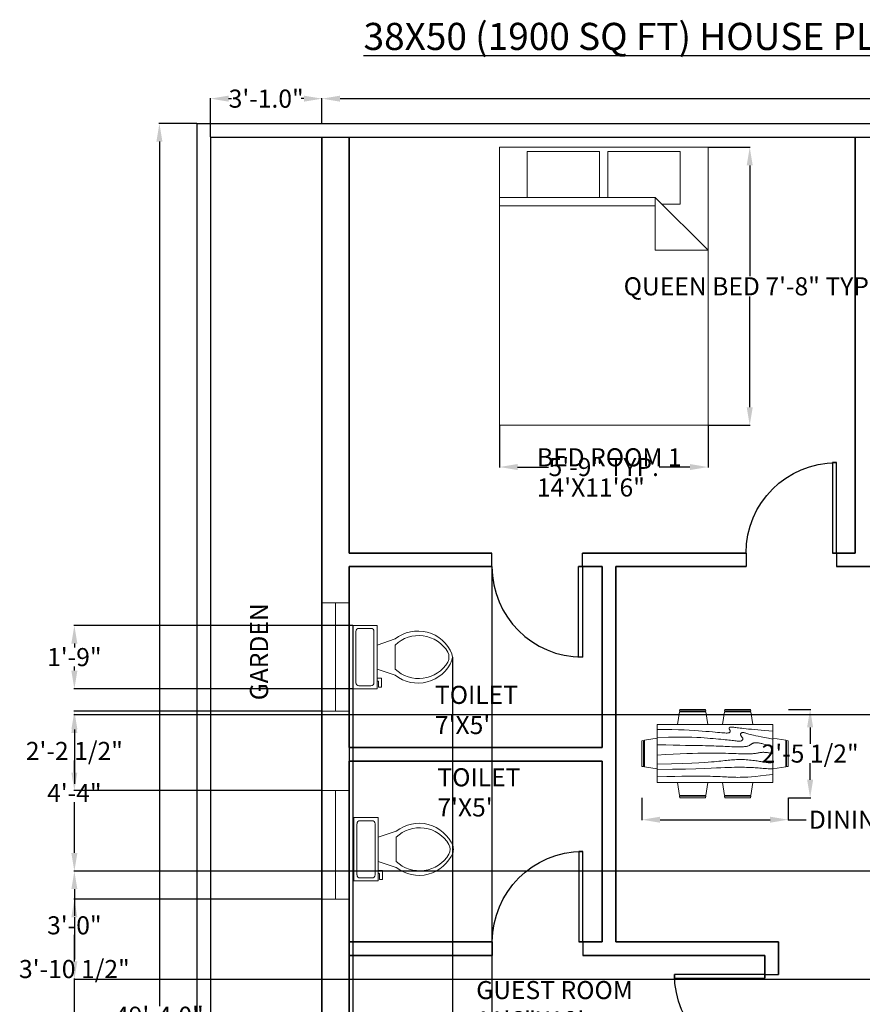
# Model space of a CAD drawing. Units: inches. Extents: x 889 to 1449, y 3224 to 3899.
# Tile 3 of 4: x 889 to 1169, y 3565 to 3892. Entities that reach past the tile are written whole.
import ezdxf

# ---------------------------------------------------------------- set-up
doc = ezdxf.new("R2010")
doc.units = ezdxf.units.IN
doc.header["$MEASUREMENT"] = 0
for name, color, linetype, lineweight in [('A-ANNO-DIMS', 2, 'Continuous', 18), ('A-ANNO-TEXT', 7, 'Continuous', 25), ('A-AREA-IDEN', 7, 'Continuous', 18), ('A-DOOR', 4, 'Continuous', 25), ('A-FLOR-FIXT', 9, 'Continuous', 18), ('A-FURN', 8, 'Continuous', 18), ('A-GLAZ', 4, 'Continuous', 18), ('A-WALL', 7, 'Continuous', 35), ('C-PROP', 7, 'Continuous', 25)]:
    doc.layers.add(name, color=color, linetype=linetype, lineweight=lineweight)
doc.styles.get("Standard").update_dxf_attribs({"font": 'arial.ttf'})
doc.dimstyles.get("Standard").update_dxf_attribs({"dimtxt": 6, "dimasz": 6, "dimexe": 0.18, "dimexo": 0.0625, "dimgap": 0.09, "dimtad": 0, "dimtih": 1, "dimtoh": 1, "dimdec": 1, "dimzin": 0, "dimdsep": 46, "dimlunit": 3, "dimtxsty": 'Standard', "dimcen": 0.09, "dimadec": 0, "dimazin": 0, "dimtfac": 1, "dimtdec": 1, "dimtofl": 0, "dimtmove": 0, "dimatfit": 3, "dimfxl": 1, "dimtolj": 1, "dimtzin": 0, "dimarcsym": 0})

# ---------------------------------------------------------------- blocks, each defined once
blk = doc.blocks.new('*U2')
for p, q in [((0, 0), (0, -6)), ((40, 0), (40, -6))]:
    blk.add_line(p, q)
blk.add_lwpolyline([(0, 0), (0, 40), (1.75, 40), (1.75, 0)], close=True)
blk.add_arc((0, 0), 40, 0, 90)
blk = doc.blocks.new('Dining Set - 36 x 72 in.')
for p, q in [((-22.2343, 26.00059), (-23.4847, 17.99762)), ((-22.2304, 26), (-5.7608, 26)), ((-22, 27.5), (-22.1562, 26.50042)), ((-5.8416, 26.5), (-22.1534, 26.5)), ((-22, 27.5), (-6, 27.5)), ((-5.8437, 26.49966), (-6, 27.5)), ((-4.5152, 17.99762), (-5.7655, 25.99926)), ((5.7657, 26.00059), (4.5153, 17.99762)), ((5.7696, 26), (22.2392, 26)), ((6, 27.5), (5.8438, 26.50042)), ((22.1584, 26.5), (5.8466, 26.5)), ((6, 27.5), (22, 27.5)), ((22.1563, 26.49966), (22, 27.5)), ((23.4848, 17.99762), (22.2345, 25.99926)), ((36, 18), (-36, 18)), ((-36, 18), (-36, -18)), ((36, -18), (36, 18)), ((-45.5, 8), (-44.5004, 8.15617)), ((-45.5, 8), (-45.5, -8)), ((-44.5, -8.15843), (-44.5, 8.15338)), ((-44.0006, 8.23428), (-35.9976, 9.48474)), ((-44, 8.23041), (-44, -8.23915)), ((44.0006, 8.23428), (35.9976, 9.48474)), ((44, 8.23041), (44, -8.23915)), ((44.5, -8.15843), (44.5, 8.15338)), ((45.5, 8), (44.5005, 8.15617)), ((45.5, 8), (45.5, -8)), ((-44.4997, -8.15631), (-45.5, -8)), ((-35.9976, -9.48476), (-43.9993, -8.2345)), ((35.9976, -9.48476), (43.9993, -8.2345)), ((44.4997, -8.15631), (45.5, -8)), ((-36, -18), (36, -18)), ((-22.2343, -26.0006), (-23.4847, -17.99762)), ((-4.5152, -17.99762), (-5.7655, -25.99928)), ((5.7657, -26.0006), (4.5153, -17.99762)), ((23.4848, -17.99762), (22.2345, -25.99928)), ((-22.2304, -26), (-5.7608, -26)), ((-22, -27.5), (-22.1562, -26.50044)), ((-5.8416, -26.5), (-22.1534, -26.5)), ((-22, -27.5), (-6, -27.5)), ((-5.8437, -26.49967), (-6, -27.5)), ((5.7696, -26), (22.2392, -26)), ((6, -27.5), (5.8438, -26.50044)), ((22.1584, -26.5), (5.8466, -26.5)), ((6, -27.5), (22, -27.5)), ((22.1563, -26.49967), (22, -27.5))]:
    blk.add_line(p, q)
for points in [[(-36, 15), (-31.1772, 14.97754), (-26.8079, 14.91406), (-22.8538, 14.81543), (-19.276, 14.6875), (-16.0362, 14.53613), (-13.0957, 14.36718), (-10.4159, 14.18652), (-7.9583, 14), (-5.6904, 13.81315), (-3.6035, 13.63021), (-1.6954, 13.45508), (0.0365, 13.29166), (1.5945, 13.14388), (2.9811, 13.01562), (4.1988, 12.9108), (5.25, 12.83333), (6.1393, 12.78613), (6.8802, 12.76823), (7.4883, 12.77767), (7.9792, 12.8125), (8.3685, 12.87077), (8.6719, 12.95052), (8.9049, 13.0498), (9.0833, 13.16666), (9.2205, 13.29899), (9.3216, 13.44401), (9.3895, 13.59879), (9.4271, 13.76041), (9.4373, 13.92594), (9.4232, 14.09245), (9.3875, 14.257), (9.3333, 14.41666), (9.2638, 14.56917), (9.1836, 14.71484), (9.0975, 14.85465), (9.0104, 14.98958), (8.9272, 15.1206), (8.8529, 15.2487), (8.7922, 15.37483), (8.75, 15.5), (8.7305, 15.62467), (8.7344, 15.74739), (8.7617, 15.86621), (8.8125, 15.97916), (8.8867, 16.08431), (8.9844, 16.17968), (9.1055, 16.26334), (9.25, 16.33333), (9.4189, 16.38802), (9.6172, 16.42708), (9.8506, 16.45052), (10.125, 16.45833), (10.4463, 16.45052), (10.8203, 16.42708), (11.2529, 16.38802), (11.75, 16.33333), (12.3184, 16.26318), (12.9694, 16.17838), (13.7151, 16.07991), (14.5677, 15.96875), (15.5395, 15.84586), (16.6426, 15.71224), (17.8893, 15.56884), (19.2917, 15.41666), (20.859, 15.25667), (22.5879, 15.08984), (24.4721, 14.91715), (26.5052, 14.73958), (28.6809, 14.5581), (30.9929, 14.3737), (33.4347, 14.18733), (36, 14)], [(-36, 10), (-28.9766, 10.14274), (-23.1725, 10.20442), (-18.4241, 10.19775), (-14.5677, 10.13541), (-11.4399, 10.03011), (-8.877, 9.89453), (-6.7154, 9.74137), (-4.7917, 9.58333), (-2.9698, 9.43082), (-1.2246, 9.28515), (0.4415, 9.14534), (2.026, 9.01041), (3.5266, 8.87939), (4.9408, 8.7513), (6.266, 8.62516), (7.5, 8.5), (8.6411, 8.37549), (9.6914, 8.2539), (10.6538, 8.13818), (11.5312, 8.03125), (12.3267, 7.93603), (13.043, 7.85547), (13.6831, 7.79248), (14.25, 7.75), (14.7471, 7.7303), (15.1797, 7.73307), (15.5537, 7.75732), (15.875, 7.80208), (16.1494, 7.86637), (16.3828, 7.94922), (16.5811, 8.04964), (16.75, 8.16666), (16.8944, 8.29915), (17.0143, 8.44531), (17.1089, 8.60319), (17.1771, 8.77083), (17.218, 8.94629), (17.2305, 9.1276), (17.2137, 9.31282), (17.1667, 9.5), (17.0895, 9.6875), (16.987, 9.875), (16.8649, 10.0625), (16.7292, 10.25), (16.5856, 10.4375), (16.4401, 10.625), (16.2985, 10.8125), (16.1667, 11), (16.05, 11.18733), (15.9518, 11.3737), (15.8752, 11.5581), (15.8229, 11.73958), (15.798, 11.91715), (15.8034, 12.08984), (15.842, 12.25667), (15.9167, 12.41666), (16.0295, 12.56836), (16.1784, 12.70833), (16.3605, 12.83268), (16.5729, 12.9375), (16.8127, 13.01888), (17.0768, 13.07291), (17.3625, 13.0957), (17.6667, 13.08333), (17.9894, 13.03312), (18.3418, 12.94726), (18.7382, 12.82918), (19.1927, 12.68229), (19.7195, 12.51001), (20.3327, 12.31575), (21.0465, 12.10294), (21.875, 11.875), (22.8357, 11.63354), (23.959, 11.37304), (25.2786, 11.08618), (26.8282, 10.76562), (28.6414, 10.40405), (30.752, 9.99414), (33.1936, 9.52856), (36, 9)], [(-36, 5.5), (-30.7157, 5.3348), (-26.069, 5.20963), (-21.9946, 5.11767), (-18.4271, 5.05208), (-15.3009, 5.00602), (-12.5508, 4.97265), (-10.1112, 4.94515), (-7.9167, 4.91666), (-5.909, 4.88167), (-4.0586, 4.83984), (-2.3429, 4.79215), (-0.7396, 4.73958), (0.7739, 4.6831), (2.22, 4.6237), (3.6213, 4.56233), (5, 4.5), (6.373, 4.43782), (7.7344, 4.3776), (9.0723, 4.32129), (10.375, 4.27083), (11.6309, 4.22819), (12.8281, 4.19531), (13.9551, 4.17415), (15, 4.16666), (15.954, 4.17448), (16.819, 4.19791), (17.6001, 4.23698), (18.3021, 4.29166), (18.9299, 4.36198), (19.4883, 4.44791), (19.9823, 4.54948), (20.4167, 4.66666), (20.7969, 4.79899), (21.1302, 4.94401), (21.4245, 5.09879), (21.6875, 5.26041), (21.9271, 5.42594), (22.1511, 5.59245), (22.3672, 5.757), (22.5834, 5.91666), (22.8065, 6.06868), (23.0404, 6.21093), (23.2879, 6.34147), (23.5521, 6.45833), (23.8358, 6.55957), (24.142, 6.64323), (24.4735, 6.70735), (24.8334, 6.75), (25.2235, 6.76969), (25.642, 6.76692), (26.0858, 6.74267), (26.5521, 6.69791), (27.0379, 6.63362), (27.5404, 6.55078), (28.0565, 6.45036), (28.5834, 6.33333), (29.1242, 6.19987), (29.7071, 6.04687), (30.3661, 5.87044), (31.1354, 5.66666), (32.0493, 5.43164), (33.142, 5.16146), (34.4475, 4.85221), (36, 4.5)], [(-36, -1), (-30.7915, -0.6591), (-26.0195, -0.38216), (-21.6519, -0.16284), (-17.6563, 0.00521), (-14.0005, 0.12833), (-10.6523, 0.21289), (-7.5796, 0.26522), (-4.75, 0.29166), (-2.134, 0.29793), (0.2878, 0.28711), (2.5317, 0.26163), (4.6146, 0.22396), (6.5529, 0.17651), (8.3633, 0.12174), (10.0623, 0.06209), (11.6667, 0), (13.1899, -0.06201), (14.6341, -0.1211), (15.9982, -0.17432), (17.2813, -0.21875), (18.4823, -0.25147), (19.6003, -0.26953), (20.6343, -0.27002), (21.5834, -0.25), (22.4481, -0.20768), (23.2357, -0.14584), (23.9549, -0.06836), (24.6146, 0.02083), (25.2235, 0.11784), (25.7904, 0.21875), (26.3241, 0.31966), (26.8334, 0.41666), (27.3265, 0.50618), (27.8099, 0.58593), (28.2894, 0.65397), (28.7709, 0.70833), (29.2601, 0.74707), (29.763, 0.76823), (30.2855, 0.76985), (30.8334, 0.75), (31.4088, 0.70784), (31.9994, 0.64713), (32.589, 0.57275), (33.1615, 0.48958), (33.7008, 0.4025), (34.1908, 0.3164), (34.6153, 0.23616), (34.9584, 0.16666), (35.2099, 0.11165), (35.3848, 0.07031), (35.504, 0.04069), (35.5886, 0.02083), (35.6594, 0.00879), (35.7377, 0.0026), (35.8442, 0.00032), (36, 0)], [(-36, -6.5), (-27.1843, -6.31267), (-20.084, -6.1263), (-14.469, -5.9419), (-10.1094, -5.76042), (-6.7752, -5.58285), (-4.2363, -5.41016), (-2.2629, -5.24333), (-0.625, -5.08334), (0.8708, -4.93099), (2.2715, -4.78646), (3.5872, -4.64974), (4.8281, -4.52084), (6.0046, -4.39974), (7.127, -4.28646), (8.2053, -4.18099), (9.25, -4.08334), (10.2705, -3.99382), (11.2734, -3.91407), (12.2647, -3.84603), (13.25, -3.79167), (14.2354, -3.75293), (15.2266, -3.73177), (16.2295, -3.73015), (17.25, -3.75), (18.2912, -3.79248), (19.3451, -3.85547), (20.4009, -3.93604), (21.4479, -4.03125), (22.4754, -4.13819), (23.4727, -4.25391), (24.4289, -4.37549), (25.3334, -4.5), (26.1785, -4.62492), (26.9694, -4.74935), (27.7145, -4.87281), (28.4219, -4.99479), (29.1, -5.11483), (29.7572, -5.23242), (30.4016, -5.34709), (31.0417, -5.45834), (31.6837, -5.56437), (32.3262, -5.65821), (32.9658, -5.73153), (33.599, -5.77604), (34.2224, -5.78345), (34.8327, -5.74545), (35.4264, -5.65373), (36, -5.5)], [(-36, -10), (-26.4022, -9.81299), (-18.4675, -9.62891), (-11.9839, -9.45069), (-6.7396, -9.28125), (-2.5226, -9.12354), (0.8789, -8.98047), (3.6769, -8.85498), (6.0833, -8.75), (8.2767, -8.66765), (10.3021, -8.60677), (12.1712, -8.56543), (13.8958, -8.54167), (15.4876, -8.53353), (16.9583, -8.53907), (18.3197, -8.55632), (19.5834, -8.58334), (20.7616, -8.61841), (21.8685, -8.66081), (22.9188, -8.71004), (23.9271, -8.76563), (24.9081, -8.82707), (25.8763, -8.89388), (26.8465, -8.96558), (27.8334, -9.04167), (28.8474, -9.12118), (29.8828, -9.20117), (30.93, -9.27824), (31.9792, -9.34896), (33.0205, -9.40991), (34.0443, -9.45768), (35.0407, -9.48885), (36, -9.5)], [(-36, -14.5), (-30.0881, -14.33513), (-25.0332, -14.21224), (-20.7312, -14.12647), (-17.0781, -14.07292), (-13.97, -14.04671), (-11.3027, -14.04297), (-8.9724, -14.05681), (-6.875, -14.08334), (-4.9224, -14.11833), (-3.0905, -14.16016), (-1.3709, -14.20785), (0.2448, -14.26042), (1.7647, -14.3169), (3.1973, -14.3763), (4.5507, -14.43767), (5.8333, -14.5), (7.0554, -14.5621), (8.235, -14.62175), (9.3922, -14.67652), (10.5469, -14.72396), (11.7192, -14.76164), (12.929, -14.78711), (14.1965, -14.79794), (15.5417, -14.79167), (16.9933, -14.76424), (18.6152, -14.70508), (20.4804, -14.60197), (22.6615, -14.44271), (25.2312, -14.21509), (28.2624, -13.9069), (31.8277, -13.50594), (36, -13)]]:
    blk.add_lwpolyline(points)
blk = doc.blocks.new('Bed - Queen')
for p, q in [((0, -80.00003), (0, 0)), ((0, 0), (59.99999, 0)), ((59.99999, 0), (59.99999, -80.00003)), ((7.99999, -1.2), (28.79998, -1.2)), ((7.99999, -14.4), (7.99999, -1.2)), ((28.79998, -1.2), (28.79998, -14.4)), ((31.19999, -1.2), (51.99999, -1.2)), ((31.19999, -14.4), (31.19999, -1.2)), ((51.99999, -1.2), (51.99999, -16.4)), ((0, -14.4), (44.8, -14.4)), ((44.8, -16.8), (0, -16.8)), ((59.99999, -29.6), (44.8, -14.4)), ((44.8, -14.4), (44.8, -29.6)), ((51.99999, -16.4), (46.79936, -16.4)), ((44.8, -29.6), (59.99999, -29.6)), ((59.99999, -80.00003), (0, -80.00003))]:
    blk.add_line(p, q)
blk = doc.blocks.new('*U15')
for p, q in [((9.5, -6), (9.5, -2)), ((-10, -8.5), (-8, -8.5)), ((-10, -9.5), (-10, -8.5)), ((-7, -9.5), (-10, -9.5)), ((-8, -8.5), (-8, -8)), ((-7, -8), (-7, -9.5)), ((-4, -8), (-6, -14)), ((4, -8), (6, -14)), ((4, -14), (-4, -14))]:
    blk.add_line(p, q)
blk.add_lwpolyline([(10.5, -8), (10.5, 0), (-10.5, 0), (-10.5, -8)], close=True)
for points in [[(-9.5, -2), (-9.5, -6)], [(8.5, -1), (-8.5, -1)], [(-8.5, -7), (8.5, -7)]]:
    blk.add_lwpolyline(points)
for centre, radius, start, end in [((-8.62, -1.88), 0.884, 81.8699, 188.1301), ((8.62, -1.88), 0.884, 351.8699, 98.1301), ((-8.62, -6.12), 0.884, 171.8699, 278.1301), ((8.62, -6.12), 0.884, 261.8699, 8.1301), ((3.52, -21.58), 12.17, 141.4691, 247.9714), ((4.2, -21.82), 11.33, 136.3677, 238.9468), ((-3.52, -21.58), 12.17, 292.0284, 38.5307), ((-4.2, -21.82), 11.33, 301.053, 43.6321), ((0, -27.88), 4, 245.7318, 294.2682), ((0, -29), 4, 254.8605, 285.1395)]:
    blk.add_arc(centre, radius, start, end)
blk = doc.blocks.new('*D17')
at = {"layer": 'A-ANNO-DIMS', "color": 0, "lineweight": -2, "transparency": 16777216}
for p, q in [((952.45, 3852.92), (952.45, 3865.8)), ((958.45, 3865.62), (959.39, 3865.62)), ((983.45, 3865.62), (982.5, 3865.62)), ((989.45, 3857.42), (989.45, 3865.8))]:
    blk.add_line(p, q, dxfattribs=at)
at = {"layer": 'A-ANNO-DIMS', "color": 0, "transparency": 16777216}
for points in [[(958.45, 3866.62), (958.45, 3864.62), (952.45, 3865.62)], [(983.45, 3866.62), (983.45, 3864.62), (989.45, 3865.62)]]:
    blk.add_solid(points, dxfattribs=at)
at = {"layer": 'Defpoints', "color": 0, "transparency": 16777216}
for p in [(989.45, 3865.62), (989.45, 3857.35), (952.45, 3852.85)]:
    blk.add_point(p, dxfattribs=at)
at = {"layer": 'A-ANNO-DIMS', "color": 0, "transparency": 16777216, "insert": (970.95, 3865.62), "char_height": 6, "attachment_point": 5}
blk.add_mtext('\\A1;3\'-1.0"', dxfattribs=at)
blk = doc.blocks.new('*D18')
at = {"layer": 'A-ANNO-DIMS', "color": 0, "lineweight": -2, "transparency": 16777216}
for p, q in [((989.45, 3857.42), (989.45, 3865.8)), ((995.45, 3865.62), (1181.06, 3865.62)), ((1394.45, 3865.62), (1208.83, 3865.62)), ((1400.45, 3857.42), (1400.45, 3865.8))]:
    blk.add_line(p, q, dxfattribs=at)
at = {"layer": 'A-ANNO-DIMS', "color": 0, "transparency": 16777216}
for points in [[(995.45, 3866.62), (995.45, 3864.62), (989.45, 3865.62)], [(1394.45, 3866.62), (1394.45, 3864.62), (1400.45, 3865.62)]]:
    blk.add_solid(points, dxfattribs=at)
at = {"layer": 'Defpoints', "color": 0, "transparency": 16777216}
for p in [(1400.45, 3865.62), (989.45, 3857.35), (1400.45, 3857.35)]:
    blk.add_point(p, dxfattribs=at)
at = {"layer": 'A-ANNO-DIMS', "color": 0, "transparency": 16777216, "insert": (1194.95, 3865.62), "char_height": 6, "attachment_point": 5}
blk.add_mtext('\\A1;34\'-3.0"', dxfattribs=at)
blk = doc.blocks.new('*D19')
at = {"layer": 'A-ANNO-DIMS', "color": 0, "lineweight": -2, "transparency": 16777216}
for p, q in [((947.88, 3857.35), (935.33, 3857.35)), ((935.51, 3851.35), (935.51, 3564.51)), ((935.51, 3271.35), (935.51, 3558.2)), ((947.88, 3265.35), (935.33, 3265.35))]:
    blk.add_line(p, q, dxfattribs=at)
at = {"layer": 'A-ANNO-DIMS', "color": 0, "transparency": 16777216}
for points in [[(934.51, 3851.35), (936.51, 3851.35), (935.51, 3857.35)], [(934.51, 3271.35), (936.51, 3271.35), (935.51, 3265.35)]]:
    blk.add_solid(points, dxfattribs=at)
at = {"layer": 'Defpoints', "color": 0, "transparency": 16777216}
for p in [(947.95, 3857.35), (935.51, 3265.35), (947.95, 3265.35)]:
    blk.add_point(p, dxfattribs=at)
at = {"layer": 'A-ANNO-DIMS', "color": 0, "transparency": 16777216, "insert": (935.51, 3561.35), "char_height": 6, "attachment_point": 5}
blk.add_mtext('\\A1;49\'-4.0"', dxfattribs=at)
blk = doc.blocks.new('WIN-36IN')
blk.add_line((4.5, 36), (4.5, 0))
blk.add_lwpolyline([(9, 36), (9, 0), (0, 0), (0, 36)], close=True)
blk = doc.blocks.new('*D30')
at = {"layer": 'A-ANNO-DIMS', "color": 0, "lineweight": -2, "transparency": 16777216}
for p, q in [((1117.62, 3849.48), (1131.58, 3849.48)), ((1131.4, 3843.48), (1131.4, 3806.74)), ((1131.4, 3763.24), (1131.4, 3799.99)), ((1117.62, 3757.24), (1131.58, 3757.24))]:
    blk.add_line(p, q, dxfattribs=at)
at = {"layer": 'A-ANNO-DIMS', "color": 0, "transparency": 16777216}
for points in [[(1130.4, 3843.48), (1132.4, 3843.48), (1131.4, 3849.48)], [(1130.4, 3763.24), (1132.4, 3763.24), (1131.4, 3757.24)]]:
    blk.add_solid(points, dxfattribs=at)
at = {"layer": 'Defpoints', "color": 0, "transparency": 16777216}
for p in [(1117.56, 3849.48), (1131.4, 3849.48), (1117.56, 3757.24)]:
    blk.add_point(p, dxfattribs=at)
at = {"layer": 'A-ANNO-DIMS', "color": 0, "transparency": 16777216, "insert": (1131.4, 3803.36), "char_height": 6, "attachment_point": 5}
blk.add_mtext('\\A1;QUEEN BED 7\'-8" TYP.', dxfattribs=at)
blk = doc.blocks.new('*D31')
at = {"layer": 'A-ANNO-DIMS', "color": 0, "lineweight": -2, "transparency": 16777216}
for p, q in [((1048.38, 3757.18), (1048.38, 3743.22)), ((1117.56, 3757.18), (1117.56, 3743.22)), ((1054.38, 3743.4), (1064.59, 3743.4)), ((1111.56, 3743.4), (1101.35, 3743.4))]:
    blk.add_line(p, q, dxfattribs=at)
at = {"layer": 'A-ANNO-DIMS', "color": 0, "transparency": 16777216}
for points in [[(1054.38, 3744.4), (1054.38, 3742.4), (1048.38, 3743.4)], [(1111.56, 3744.4), (1111.56, 3742.4), (1117.56, 3743.4)]]:
    blk.add_solid(points, dxfattribs=at)
at = {"layer": 'Defpoints', "color": 0, "transparency": 16777216}
for p in [(1048.38, 3757.24), (1117.56, 3757.24), (1117.56, 3743.4)]:
    blk.add_point(p, dxfattribs=at)
at = {"layer": 'A-ANNO-DIMS', "color": 0, "transparency": 16777216, "insert": (1082.97, 3743.4), "char_height": 6, "attachment_point": 5}
blk.add_mtext('\\A1;5\'-9" TYP.', dxfattribs=at)
blk = doc.blocks.new('*D36')
at = {"layer": 'A-ANNO-DIMS', "color": 0, "lineweight": -2, "transparency": 16777216}
for p, q in [((1095.64, 3633.61), (1095.64, 3626.21)), ((1144.17, 3633.61), (1144.17, 3626.21)), ((1101.64, 3626.39), (1138.17, 3626.39)), ((1144.17, 3626.39), (1150.17, 3626.39))]:
    blk.add_line(p, q, dxfattribs=at)
at = {"layer": 'A-ANNO-DIMS', "color": 0, "transparency": 16777216}
for points in [[(1101.64, 3627.39), (1101.64, 3625.39), (1095.64, 3626.39)], [(1138.17, 3627.39), (1138.17, 3625.39), (1144.17, 3626.39)]]:
    blk.add_solid(points, dxfattribs=at)
at = {"layer": 'Defpoints', "color": 0, "transparency": 16777216}
for p in [(1095.64, 3633.67), (1144.17, 3633.67), (1144.17, 3626.39)]:
    blk.add_point(p, dxfattribs=at)
at = {"layer": 'A-ANNO-DIMS', "color": 0, "transparency": 16777216, "insert": (1190.23, 3626.39), "char_height": 6, "attachment_point": 5}
blk.add_mtext('\\A1;DINING SET 4\'-0 1/2"', dxfattribs=at)
blk = doc.blocks.new('*D37')
at = {"layer": 'A-ANNO-DIMS', "color": 0, "lineweight": -2, "transparency": 16777216}
for p, q in [((1144.24, 3663.01), (1151.63, 3663.01)), ((1151.45, 3657.01), (1151.45, 3651.53)), ((1151.45, 3639.67), (1151.45, 3645.15)), ((1144.24, 3633.67), (1151.63, 3633.67))]:
    blk.add_line(p, q, dxfattribs=at)
at = {"layer": 'A-ANNO-DIMS', "color": 0, "transparency": 16777216}
for points in [[(1150.45, 3657.01), (1152.45, 3657.01), (1151.45, 3663.01)], [(1150.45, 3639.67), (1152.45, 3639.67), (1151.45, 3633.67)]]:
    blk.add_solid(points, dxfattribs=at)
at = {"layer": 'Defpoints', "color": 0, "transparency": 16777216}
for p in [(1144.17, 3663.01), (1151.45, 3663.01), (1144.17, 3633.67)]:
    blk.add_point(p, dxfattribs=at)
at = {"layer": 'A-ANNO-DIMS', "color": 0, "transparency": 16777216, "insert": (1151.45, 3648.34), "char_height": 6, "attachment_point": 5}
blk.add_mtext('\\A1;2\'-5 1/2"', dxfattribs=at)
blk = doc.blocks.new('*D53')
at = {"layer": 'A-ANNO-DIMS', "color": 0, "lineweight": -2, "transparency": 16777216}
for p, q in [((989.38, 3600.04), (907.11, 3600.04)), ((907.29, 3594.04), (907.29, 3580.05)), ((907.29, 3559.66), (907.29, 3573.66)), ((989.38, 3553.66), (907.11, 3553.66))]:
    blk.add_line(p, q, dxfattribs=at)
at = {"layer": 'A-ANNO-DIMS', "color": 0, "transparency": 16777216}
for points in [[(906.29, 3594.04), (908.29, 3594.04), (907.29, 3600.04)], [(906.29, 3559.66), (908.29, 3559.66), (907.29, 3553.66)]]:
    blk.add_solid(points, dxfattribs=at)
at = {"layer": 'Defpoints', "color": 0, "transparency": 16777216}
for p in [(907.29, 3600.04), (989.45, 3600.04), (989.45, 3553.66)]:
    blk.add_point(p, dxfattribs=at)
at = {"layer": 'A-ANNO-DIMS', "color": 0, "transparency": 16777216, "insert": (907.29, 3576.85), "char_height": 6, "attachment_point": 5}
blk.add_mtext('\\A1;3\'-10 1/2"', dxfattribs=at)
blk = doc.blocks.new('*D54')
at = {"layer": 'A-ANNO-DIMS', "color": 0, "lineweight": -2, "transparency": 16777216}
for p, q in [((989.38, 3662.35), (907.11, 3662.35)), ((907.29, 3656.35), (907.29, 3652.39)), ((907.29, 3642.04), (907.29, 3646)), ((989.38, 3636.04), (907.11, 3636.04))]:
    blk.add_line(p, q, dxfattribs=at)
at = {"layer": 'A-ANNO-DIMS', "color": 0, "transparency": 16777216}
for points in [[(906.29, 3656.35), (908.29, 3656.35), (907.29, 3662.35)], [(906.29, 3642.04), (908.29, 3642.04), (907.29, 3636.04)]]:
    blk.add_solid(points, dxfattribs=at)
at = {"layer": 'Defpoints', "color": 0, "transparency": 16777216}
for p in [(907.29, 3662.35), (989.45, 3662.35), (989.45, 3636.04)]:
    blk.add_point(p, dxfattribs=at)
at = {"layer": 'A-ANNO-DIMS', "color": 0, "transparency": 16777216, "insert": (907.29, 3649.2), "char_height": 6, "attachment_point": 5}
blk.add_mtext('\\A1;2\'-2 1/2"', dxfattribs=at)
blk = doc.blocks.new('*D58')
at = {"layer": 'A-ANNO-DIMS', "color": 0, "lineweight": -2, "transparency": 16777216}
for p, q in [((1197.23, 3609.35), (907.11, 3609.35)), ((907.29, 3603.35), (907.29, 3594.51)), ((907.29, 3579.35), (907.29, 3588.2)), ((1197.23, 3573.35), (907.11, 3573.35))]:
    blk.add_line(p, q, dxfattribs=at)
at = {"layer": 'A-ANNO-DIMS', "color": 0, "transparency": 16777216}
for points in [[(906.29, 3603.35), (908.29, 3603.35), (907.29, 3609.35)], [(906.29, 3579.35), (908.29, 3579.35), (907.29, 3573.35)]]:
    blk.add_solid(points, dxfattribs=at)
at = {"layer": 'Defpoints', "color": 0, "transparency": 16777216}
for p in [(907.29, 3609.35), (1197.3, 3609.35), (1197.3, 3573.35)]:
    blk.add_point(p, dxfattribs=at)
at = {"layer": 'A-ANNO-DIMS', "color": 0, "transparency": 16777216, "insert": (907.29, 3591.35), "char_height": 6, "attachment_point": 5}
blk.add_mtext('\\A1;3\'-0"', dxfattribs=at)
blk = doc.blocks.new('*D61')
at = {"layer": 'A-ANNO-DIMS', "color": 0, "lineweight": -2, "transparency": 16777216}
for p, q in [((1298.56, 3661.14), (907.11, 3661.14)), ((907.29, 3655.14), (907.29, 3638.34)), ((907.29, 3615.35), (907.29, 3632.16)), ((1298.56, 3609.35), (907.11, 3609.35))]:
    blk.add_line(p, q, dxfattribs=at)
at = {"layer": 'A-ANNO-DIMS', "color": 0, "transparency": 16777216}
for points in [[(906.29, 3655.14), (908.29, 3655.14), (907.29, 3661.14)], [(906.29, 3615.35), (908.29, 3615.35), (907.29, 3609.35)]]:
    blk.add_solid(points, dxfattribs=at)
at = {"layer": 'Defpoints', "color": 0, "transparency": 16777216}
for p in [(907.29, 3661.14), (1298.62, 3661.14), (1298.62, 3609.35)]:
    blk.add_point(p, dxfattribs=at)
at = {"layer": 'A-ANNO-DIMS', "color": 0, "transparency": 16777216, "insert": (907.29, 3635.25), "char_height": 6, "attachment_point": 5}
blk.add_mtext('\\A1;4\'-4"', dxfattribs=at)
blk = doc.blocks.new('*D62')
at = {"layer": 'A-ANNO-DIMS', "color": 0, "lineweight": -2, "transparency": 16777216}
for p, q in [((998.45, 3710.29), (998.45, 3232.74)), ((1045.87, 3710.29), (1045.87, 3232.74)), ((1004.45, 3232.92), (1004.77, 3232.92)), ((1039.87, 3232.92), (1039.54, 3232.92))]:
    blk.add_line(p, q, dxfattribs=at)
at = {"layer": 'A-ANNO-DIMS', "color": 0, "transparency": 16777216}
for points in [[(1004.45, 3233.92), (1004.45, 3231.92), (998.45, 3232.92)], [(1039.87, 3233.92), (1039.87, 3231.92), (1045.87, 3232.92)]]:
    blk.add_solid(points, dxfattribs=at)
at = {"layer": 'Defpoints', "color": 0, "transparency": 16777216}
for p in [(998.45, 3710.35), (1045.87, 3710.35), (1045.87, 3232.92)]:
    blk.add_point(p, dxfattribs=at)
at = {"layer": 'A-ANNO-DIMS', "color": 0, "transparency": 16777216, "insert": (1022.16, 3232.92), "char_height": 6, "attachment_point": 5}
blk.add_mtext('\\A1;3\'-11 1/2"', dxfattribs=at)
blk = doc.blocks.new('*D63')
at = {"layer": 'A-ANNO-DIMS', "color": 0, "lineweight": -2, "transparency": 16777216}
for p, q in [((999.72, 3690.79), (999.72, 3232.74)), ((1032.72, 3680.29), (1032.72, 3232.74)), ((1005.72, 3232.92), (1008.1, 3232.92)), ((1026.72, 3232.92), (1024.33, 3232.92))]:
    blk.add_line(p, q, dxfattribs=at)
at = {"layer": 'A-ANNO-DIMS', "color": 0, "transparency": 16777216}
for points in [[(1005.72, 3233.92), (1005.72, 3231.92), (999.72, 3232.92)], [(1026.72, 3233.92), (1026.72, 3231.92), (1032.72, 3232.92)]]:
    blk.add_solid(points, dxfattribs=at)
at = {"layer": 'Defpoints', "color": 0, "transparency": 16777216}
for p in [(999.72, 3690.85), (1032.72, 3680.35), (1032.72, 3232.92)]:
    blk.add_point(p, dxfattribs=at)
at = {"layer": 'A-ANNO-DIMS', "color": 0, "transparency": 16777216, "insert": (1016.22, 3232.92), "char_height": 6, "attachment_point": 5}
blk.add_mtext('\\A1;2\'-9"', dxfattribs=at)
blk = doc.blocks.new('*D64')
at = {"layer": 'A-ANNO-DIMS', "color": 0, "lineweight": -2, "transparency": 16777216}
for p, q in [((999.65, 3690.85), (907.11, 3690.85)), ((907.29, 3684.85), (907.29, 3683.51)), ((907.29, 3675.85), (907.29, 3677.2)), ((999.65, 3669.85), (907.11, 3669.85))]:
    blk.add_line(p, q, dxfattribs=at)
at = {"layer": 'A-ANNO-DIMS', "color": 0, "transparency": 16777216}
for points in [[(906.29, 3684.85), (908.29, 3684.85), (907.29, 3690.85)], [(906.29, 3675.85), (908.29, 3675.85), (907.29, 3669.85)]]:
    blk.add_solid(points, dxfattribs=at)
at = {"layer": 'Defpoints', "color": 0, "transparency": 16777216}
for p in [(907.29, 3690.85), (999.72, 3690.85), (999.72, 3669.85)]:
    blk.add_point(p, dxfattribs=at)
at = {"layer": 'A-ANNO-DIMS', "color": 0, "transparency": 16777216, "insert": (907.29, 3680.35), "char_height": 6, "attachment_point": 5}
blk.add_mtext('\\A1;1\'-9"', dxfattribs=at)

msp = doc.modelspace()

# ---------------------------------------------------------------- linework, layer by layer
at = {"layer": 'A-WALL'}
for p, q in [((989.45, 3852.85), (989.45, 3452.35)), ((998.45, 3852.85), (998.45, 3714.85)), ((1166.45, 3852.85), (1166.45, 3714.85)), ((998.45, 3714.85), (1045.87, 3714.85)), ((1075.87, 3714.85), (1130.18, 3714.85)), ((1158.87, 3714.85), (1166.45, 3714.85)), ((998.45, 3710.35), (1045.87, 3710.35)), ((998.45, 3710.35), (998.45, 3650.35)), ((1074.56, 3710.35), (1082.45, 3710.35)), ((1082.45, 3710.35), (1082.45, 3650.35)), ((1086.95, 3710.35), (1086.95, 3585.85)), ((1086.95, 3710.35), (1130.18, 3710.35)), ((1160.18, 3710.35), (1177.21, 3710.35)), ((998.45, 3650.35), (1082.45, 3650.35)), ((998.45, 3645.85), (1082.45, 3645.85)), ((998.45, 3645.85), (998.45, 3461.35)), ((1082.45, 3645.85), (1082.45, 3585.85)), ((998.45, 3585.85), (1045.97, 3585.85)), ((1074.66, 3585.85), (1082.45, 3585.85)), ((1086.95, 3585.85), (1140.95, 3585.85)), ((1140.95, 3585.85), (1140.95, 3575.09)), ((998.45, 3581.35), (1045.97, 3581.35)), ((1075.97, 3581.35), (1136.45, 3581.35)), ((1136.45, 3581.35), (1136.45, 3573.78))]:
    msp.add_line(p, q, dxfattribs=at)
at = {"layer": 'C-PROP'}
for p, q in [((947.95, 3857.35), (1400.45, 3857.35)), ((947.95, 3857.35), (947.95, 3265.35)), ((952.45, 3852.85), (1338.95, 3852.85)), ((952.45, 3852.85), (952.45, 3269.85))]:
    msp.add_line(p, q, dxfattribs=at)

# ---------------------------------------------------------------- block references
at = {"layer": 'A-DOOR', "xscale": -0.75, "yscale": 0.75, "zscale": 0.75}
for p in [(1160.18, 3714.85), (1075.97, 3585.85)]:
    msp.add_blockref('*U2', p, dxfattribs=at)
at = {"layer": 'A-DOOR', "yscale": 0.75, "zscale": 0.75}
for p, xscale, rotation in [((1075.87, 3710.35), 0.75, 180), ((1136.45, 3575.09), -0.75, 90)]:
    msp.add_blockref('*U2', p, dxfattribs=dict(at, xscale=xscale, rotation=rotation))
at = {"layer": 'A-FLOR-FIXT', "rotation": 90}
for p in [(999.72, 3680.35), (1000.08, 3616.57)]:
    msp.add_blockref('*U15', p, dxfattribs=at)
at = {"layer": 'A-FURN'}
for name, p, xscale, yscale, zscale in [('Bed - Queen', (1048.38, 3849.48), 1.153040595648429, 1.153040595648429, 1.153040595648429), ('Dining Set - 36 x 72 in.', (1119.91, 3648.34), 0.5333426586376082, 0.5333426586376082, 0.5333426586376082)]:
    msp.add_blockref(name, p, dxfattribs=dict(at, xscale=xscale, yscale=yscale, zscale=zscale))
at = {"layer": 'A-GLAZ'}
for p in [(989.45, 3662.36), (989.45, 3600.04)]:
    msp.add_blockref('WIN-36IN', p, dxfattribs=at)

# ---------------------------------------------------------------- texts
at = {"layer": 'A-ANNO-TEXT', "insert": (1003.26, 3890.77), "char_height": 9, "attachment_point": 1}
msp.add_mtext_dynamic_manual_height_columns('{\\fArial|b1|i0|c0|p34;\\L38X50 (1900 SQ FT) HOUSE PLAN- WEST FACE- FP1317}', width=396.8668, gutter_width=1, heights=[0], dxfattribs=at)
at = {"layer": 'A-AREA-IDEN', "char_height": 6, "attachment_point": 1}
for s, insert in [('BED ROOM 1\\P14\'X11\'6"', (1060.77, 3749.62)), ("TOILET\\P7'X5'", (1026.95, 3670.81)), ("TOILET\\P7'X5'", (1027.76, 3643.46)), ('GUEST ROOM\\P11\'6"X10\'', (1040.64, 3572.87))]:
    msp.add_mtext_dynamic_manual_height_columns(s, width=93.4406, gutter_width=1, heights=[0], dxfattribs=dict(at, insert=insert))
at = {"layer": 'A-AREA-IDEN', "insert": (965.57, 3666.01), "char_height": 6, "attachment_point": 1, "rotation": 90}
msp.add_mtext_dynamic_manual_height_columns('GARDEN', width=93.4406, gutter_width=1, heights=[0], dxfattribs=at)

# ---------------------------------------------------------------- dimensions: what is measured, and where the dimension line sits
at = {"layer": 'A-ANNO-DIMS'}
for base, p1, p2, override, picture, middle in [((989.45, 3865.62), (952.45, 3852.85), (989.45, 3857.35), {"dimclrd": 0, "dimclre": 0, "dimclrt": 0}, '*D17', (970.95, 3865.62)), ((1400.45, 3865.62), (989.45, 3857.35), (1400.45, 3857.35), {"dimclrd": 0, "dimclre": 0, "dimclrt": 0, "dimtmove": 1}, '*D18', (1194.95, 3865.62)), ((1045.87, 3232.92), (998.45, 3710.35), (1045.87, 3710.35), {"dimdec": 1, "dimlfac": 1, "dimrnd": 0, "dimzin": 1, "dimdsep": 46, "dimlunit": 4, "dimfrac": 2}, '*D62', (1022.16, 3232.92)), ((1032.72, 3232.92), (999.72, 3690.85), (1032.72, 3680.35), {"dimdec": 1, "dimlfac": 1, "dimrnd": 0, "dimzin": 1, "dimdsep": 46, "dimlunit": 4, "dimfrac": 2}, '*D63', (1016.22, 3232.92))]:
    dim = msp.add_linear_dim(base=base, p1=p1, p2=p2, dimstyle='Standard', override=override, dxfattribs=at)
    dim.commit()
    dim.dimension.update_dxf_attribs({"geometry": picture, "text_midpoint": middle})
for base, p1, p2, override, picture, middle in [((935.51, 3265.35), (947.95, 3857.35), (947.95, 3265.35), {"dimclrd": 0, "dimclre": 0, "dimclrt": 0}, '*D19', (935.51, 3561.35)), ((907.29, 3690.85), (999.72, 3669.85), (999.72, 3690.85), {"dimdec": 1, "dimlfac": 1, "dimrnd": 0, "dimzin": 1, "dimdsep": 46, "dimlunit": 4, "dimfrac": 2}, '*D64', (907.29, 3680.35)), ((907.29, 3662.35), (989.45, 3636.04), (989.45, 3662.35), {"dimdec": 1, "dimlfac": 1, "dimrnd": 0, "dimzin": 1, "dimdsep": 46, "dimlunit": 4, "dimfrac": 2}, '*D54', (907.29, 3649.2)), ((1151.45, 3663.01), (1144.17, 3633.67), (1144.17, 3663.01), {"dimdec": 1, "dimlfac": 1, "dimrnd": 0, "dimzin": 1, "dimdsep": 46, "dimlunit": 4, "dimfrac": 2}, '*D37', (1151.45, 3648.34)), ((907.29, 3661.14), (1298.62, 3609.35), (1298.62, 3661.14), {"dimdec": 1, "dimlfac": 1, "dimrnd": 0, "dimzin": 1, "dimdsep": 46, "dimlunit": 4, "dimfrac": 2}, '*D61', (907.29, 3635.25)), ((907.29, 3609.35), (1197.3, 3573.35), (1197.3, 3609.35), {"dimdec": 1, "dimlfac": 1, "dimrnd": 0, "dimzin": 1, "dimdsep": 46, "dimlunit": 4, "dimfrac": 2}, '*D58', (907.29, 3591.35)), ((907.29, 3600.04), (989.45, 3553.66), (989.45, 3600.04), {"dimdec": 1, "dimlfac": 1, "dimrnd": 0, "dimzin": 1, "dimdsep": 46, "dimlunit": 4, "dimfrac": 2}, '*D53', (907.29, 3576.85))]:
    dim = msp.add_linear_dim(base=base, p1=p1, p2=p2, angle=90, dimstyle='Standard', override=override, dxfattribs=at)
    dim.commit()
    dim.dimension.update_dxf_attribs({"geometry": picture, "text_midpoint": middle})
dim = msp.add_linear_dim(base=(1131.4, 3849.48), p1=(1117.56, 3757.24), p2=(1117.56, 3849.48), angle=90, text='QUEEN BED <> TYP.', dimstyle='Standard', override={"dimdec": 1, "dimlfac": 1, "dimrnd": 0, "dimzin": 1, "dimdsep": 46, "dimlunit": 4, "dimfrac": 2}, dxfattribs=at)
dim.commit()
dim.dimension.update_dxf_attribs({"geometry": '*D30', "text_midpoint": (1131.4, 3803.36)})
for base, p1, p2, text, picture, middle in [((1117.56, 3743.4), (1048.38, 3757.24), (1117.56, 3757.24), '<> TYP.', '*D31', (1082.97, 3743.4)), ((1144.17, 3626.39), (1095.64, 3633.67), (1144.17, 3633.67), 'DINING SET <>', '*D36', (1190.23, 3626.39))]:
    dim = msp.add_linear_dim(base=base, p1=p1, p2=p2, text=text, dimstyle='Standard', override={"dimdec": 1, "dimlfac": 1, "dimrnd": 0, "dimzin": 1, "dimdsep": 46, "dimlunit": 4, "dimfrac": 2}, dxfattribs=at)
    dim.commit()
    dim.dimension.update_dxf_attribs({"geometry": picture, "text_midpoint": middle})

doc.saveas('drawing.dxf')
